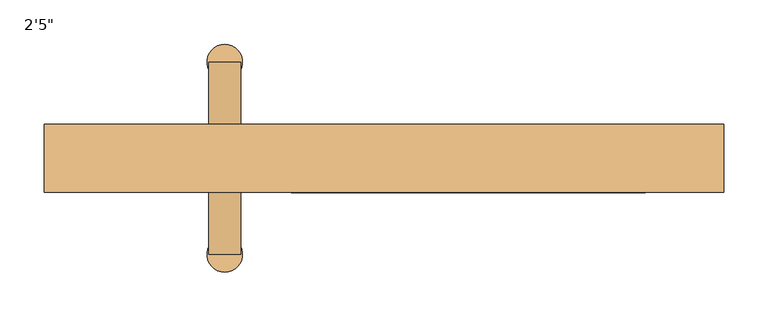
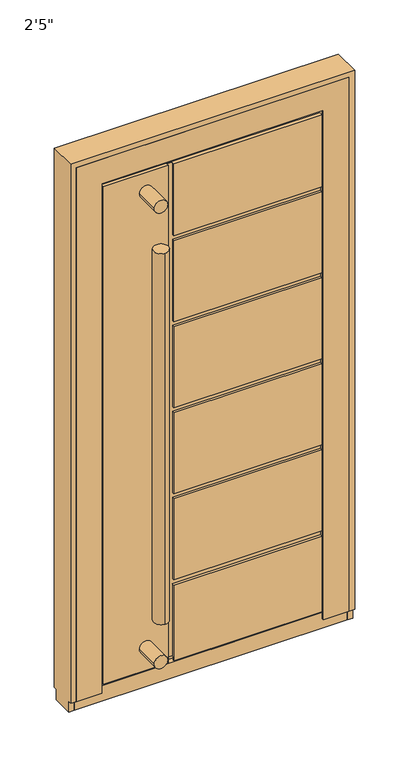
"""IFC4 building model written with IfcOpenShell, lengths in millimetres: door geometry."""

from ifc_helpers import new_model, si_unit, point, frame, frame_2d, origin, place, context, project, spatial, circle_curve, trimmed, segment, composite_curve, outline, extrude, faceted_brep, source, transform, mapped, element, save


def door_9b787682(model_context):
    return source(origin(), model_context, "Body", "SolidModel", [
        extrude(outline(composite_curve([segment(trimmed(circle_curve(frame_2d((-179.75, -90.8003001)), 20.0), [point((-179.75, -70.8003001))], [point((-179.75, -110.8003001))], False, "CARTESIAN"), True, "CONTINUOUS"), segment(trimmed(circle_curve(frame_2d((-179.75, -90.8003001)), 20.0), [point((-179.75, -110.8003001))], [point((-179.75, -70.8003001))], False, "CARTESIAN"), True, "CONTINUOUS")], self_intersect=False)), frame((0.0, 0.0, 210.0000003), z_axis=(0.0, 0.0, 1.0), x_axis=(1.0, 0.0, 0.0)), (0.0, 0.0, 1.0), 1059.0),
        extrude(outline(composite_curve([segment(trimmed(circle_curve(frame_2d((-179.75, 126.2003001)), 20.0), [point((-179.75, 146.2003001))], [point((-179.75, 106.2003001))], False, "CARTESIAN"), True, "CONTINUOUS"), segment(trimmed(circle_curve(frame_2d((-179.75, 126.2003001)), 20.0), [point((-179.75, 106.2003001))], [point((-179.75, 146.2003001))], False, "CARTESIAN"), True, "CONTINUOUS")], self_intersect=False)), frame((0.0, 0.0, 210.0000003), z_axis=(0.0, 0.0, 1.0), x_axis=(1.0, 0.0, 0.0)), (0.0, 0.0, 1.0), 1059.0),
        extrude(outline(composite_curve([segment(trimmed(circle_curve(frame_2d((89.5000003, -179.75)), 18.0), [point((89.5000003, -197.75))], [point((89.5000003, -161.75))], False, "CARTESIAN"), True, "CONTINUOUS"), segment(trimmed(circle_curve(frame_2d((89.5000003, -179.75)), 18.0), [point((89.5000003, -161.75))], [point((89.5000003, -197.75))], False, "CARTESIAN"), True, "CONTINUOUS")], self_intersect=False)), frame((0.0, -90.8, 0.0), z_axis=(0.0, 1.0, 0.0), x_axis=(0.0, 0.0, 1.0)), (0.0, 0.0, 1.0), 217.0),
        extrude(outline(composite_curve([segment(trimmed(circle_curve(frame_2d((1389.5000003, -179.75)), 18.0), [point((1389.5000003, -197.75))], [point((1389.5000003, -161.75))], False, "CARTESIAN"), True, "CONTINUOUS"), segment(trimmed(circle_curve(frame_2d((1389.5000003, -179.75)), 18.0), [point((1389.5000003, -161.75))], [point((1389.5000003, -197.75))], False, "CARTESIAN"), True, "CONTINUOUS")], self_intersect=False)), frame((0.0, -90.8, 0.0), z_axis=(0.0, 1.0, 0.0), x_axis=(0.0, 0.0, 1.0)), (0.0, 0.0, 1.0), 217.0),
        faceted_brep([(-104.75, -13.8, 255.666667), (-104.75, -13.8, 486.3333337), (294.75, -13.8, 486.3333337), (294.75, -13.8, 501.3333337), (-104.75, -13.8, 501.3333337), (-104.75, -13.8, 732.0000004), (294.75, -13.8, 732.0000004), (294.75, -13.8, 747.0000004), (-104.75, -13.8, 747.0000004), (-104.75, -13.8, 977.666667), (294.75, -13.8, 977.666667), (294.75, -13.8, 992.666667), (-104.75, -13.8, 992.666667), (-104.75, -13.8, 1223.3333337), (294.75, -13.8, 1223.3333337), (294.75, -13.8, 1238.3333337), (-104.75, -13.8, 1238.3333337), (-104.75, -13.8, 1444.0000003), (-119.75, -13.8, 1444.0000003), (-119.75, -13.8, 35.0), (-104.75, -13.8, 35.0), (-104.75, -13.8, 240.666667), (294.75, -13.8, 240.666667), (294.75, -13.8, 255.666667), (-104.75, -20.8, 255.666667), (-104.75, -20.8, 486.3333337), (294.75, -20.8, 486.3333337), (294.75, -11.7997698, 1444.0000003), (294.75, -20.8, 1444.0000003), (294.75, -20.8, 1238.3333337), (294.75, -20.8, 1223.3333337), (294.75, -20.8, 992.666667), (294.75, -20.8, 977.666667), (294.75, -20.8, 747.0000004), (294.75, -20.8, 732.0000004), (294.75, -20.8, 501.3333337), (294.75, -20.8, 255.666667), (294.75, -20.8, 240.666667), (294.75, -20.8, 24.0), (294.75, -18.8020472, 24.0), (294.75, -18.8020472, 35.0), (294.75, -11.7997698, 35.0), (-104.75, -20.8, 501.3333337), (-104.75, -20.8, 732.0000004), (-104.75, -20.8, 747.0000004), (-104.75, -20.8, 977.666667), (-119.75, -20.8, 1444.0000003), (-119.75, -20.8, 24.0), (-119.75, -18.8020472, 24.0), (-119.75, -18.8020472, 35.0), (-104.75, -18.8020472, 35.0), (-294.75, -18.8020472, 35.0), (-294.75, -11.7997698, 35.0), (-104.75, -20.8, 240.666667), (-104.75, -18.8020472, 24.0), (-104.75, -20.8, 24.0), (-294.75, -18.8020472, 24.0), (-294.75, -20.8, 24.0), (-294.75, -20.8, 1444.0000003), (-104.75, -20.8, 1223.3333337), (-104.75, -20.8, 992.666667), (-104.75, -20.8, 1444.0000003), (-104.75, -20.8, 1238.3333337), (319.75, 56.2, 10.0000003), (319.75, 53.2, 10.0000003), (-104.75, 53.2, 10.0000003), (-104.75, 56.2, 10.0000003), (-319.75, 53.2, 10.0000003), (-319.75, 56.2, 10.0000003), (-119.75, 56.2, 10.0000003), (-119.75, 53.2, 10.0000003), (319.75, 56.2, 240.666667), (319.75, 53.2, 240.666667), (319.75, 56.2, 255.666667), (319.75, 56.2, 486.3333337), (319.75, 53.2, 486.3333337), (319.75, 53.2, 255.666667), (319.75, 56.2, 747.0000004), (319.75, 56.2, 977.666667), (319.75, 53.2, 977.666667), (319.75, 53.2, 747.0000004), (319.75, 56.2, 501.3333337), (319.75, 56.2, 732.0000004), (319.75, 53.2, 732.0000004), (319.75, 53.2, 501.3333337), (319.75, 56.2, 992.666667), (319.75, 56.2, 1223.3333337), (319.75, 53.2, 1223.3333337), (319.75, 53.2, 992.666667), (319.75, 56.2, 1469.0000003), (319.75, 53.2, 1469.0000003), (319.75, 53.2, 1238.3333337), (319.75, 56.2, 1238.3333337), (304.25, 53.2, 240.666667), (304.25, 53.2, 25.5), (-104.75, 53.2, 25.5), (304.25, 53.2, 486.3333337), (304.25, 53.2, 255.666667), (304.25, 53.2, 977.666667), (304.25, 53.2, 747.0000004), (304.25, 53.2, 732.0000004), (304.25, 53.2, 501.3333337), (304.25, 53.2, 1223.3333337), (304.25, 53.2, 992.666667), (-104.75, 53.2, 1469.0000003), (-104.75, 53.2, 1453.5000003), (304.25, 53.2, 1453.5000003), (304.25, 53.2, 1238.3333337), (-304.25, 53.2, 25.5), (-304.25, 53.2, 1453.5000003), (-119.75, 53.2, 1453.5000003), (-119.75, 53.2, 1469.0000003), (-319.75, 53.2, 1469.0000003), (-119.75, 53.2, 25.5), (-104.75, 49.2, 240.666667), (-104.75, 56.2, 240.666667), (-104.75, 49.2, 25.5), (-104.75, 56.2, 255.666667), (-104.75, 56.2, 486.3333337), (-104.75, 56.2, 747.0000004), (-104.75, 56.2, 977.666667), (-104.75, 56.2, 501.3333337), (-104.75, 56.2, 732.0000004), (-104.75, 56.2, 992.666667), (-104.75, 56.2, 1223.3333337), (-104.75, 56.2, 1238.3333337), (-104.75, 56.2, 1469.0000003), (-319.75, 56.2, 1469.0000003), (-119.75, 56.2, 1469.0000003), (-119.75, 49.2, 1453.5000003), (-119.75, 49.2, 25.5), (-294.75, -11.7997698, 1444.0000003), (304.25, -11.7997698, 1453.5000003), (-304.25, -11.7997698, 1453.5000003), (-304.25, -11.7997698, 25.5), (304.25, -11.7997698, 25.5), (304.25, 49.2, 240.666667), (304.25, 49.2, 255.666667), (304.25, 49.2, 486.3333337), (304.25, 49.2, 501.3333337), (304.25, 49.2, 732.0000004), (304.25, 49.2, 747.0000004), (304.25, 49.2, 977.666667), (304.25, 49.2, 992.666667), (304.25, 49.2, 1223.3333337), (304.25, 49.2, 1238.3333337), (-104.75, 49.2, 1223.3333337), (-104.75, 49.2, 992.666667), (-104.75, 49.2, 977.666667), (-104.75, 49.2, 747.0000004), (-104.75, 49.2, 732.0000004), (-104.75, 49.2, 501.3333337), (-104.75, 49.2, 486.3333337), (-104.75, 49.2, 255.666667), (-104.75, 49.2, 1453.5000003), (-104.75, 49.2, 1238.3333337)], [[[0, 1, 2, 3, 4, 5, 6, 7, 8, 9, 10, 11, 12, 13, 14, 15, 16, 17, 18, 19, 20, 21, 22, 23]], [[1, 0, 24, 25]], [[1, 25, 26, 2]], [[27, 28, 29, 15, 14, 30, 31, 11, 10, 32, 33, 7, 6, 34, 35, 3, 2, 26, 36, 23, 22, 37, 38, 39, 40, 41]], [[42, 4, 3, 35]], [[5, 4, 42, 43]], [[5, 43, 34, 6]], [[44, 8, 7, 33]], [[9, 8, 44, 45]], [[19, 18, 46, 47, 48, 49]], [[41, 40, 50, 20, 19, 49, 51, 52]], [[53, 21, 20, 50, 54, 55]], [[21, 53, 37, 22]], [[24, 0, 23, 36]], [[40, 39, 54, 50]], [[56, 51, 49, 48]], [[39, 38, 55, 54]], [[57, 56, 48, 47]], [[33, 32, 45, 44]], [[35, 34, 43, 42]], [[36, 26, 25, 24]], [[55, 38, 37, 53]], [[58, 57, 47, 46]], [[31, 30, 59, 60]], [[28, 61, 62, 29]], [[63, 64, 65, 66]], [[67, 68, 69, 70]], [[64, 63, 71, 72]], [[73, 74, 75, 76]], [[77, 78, 79, 80]], [[81, 82, 83, 84]], [[85, 86, 87, 88]], [[89, 90, 91, 92]], [[65, 64, 72, 93, 94, 95]], [[76, 75, 96, 97]], [[80, 79, 98, 99]], [[84, 83, 100, 101]], [[88, 87, 102, 103]], [[90, 104, 105, 106, 107, 91]], [[108, 109, 110, 111, 112, 67, 70, 113]], [[114, 115, 66, 65, 95, 116]], [[63, 66, 115, 71]], [[74, 73, 117, 118]], [[78, 77, 119, 120]], [[82, 81, 121, 122]], [[86, 85, 123, 124]], [[89, 92, 125, 126]], [[68, 127, 128, 69]], [[68, 67, 112, 127]], [[129, 130, 113, 70, 69, 128, 111, 110]], [[58, 131, 52, 51, 56, 57]], [[132, 133, 134, 135], [131, 27, 41, 52]], [[106, 132, 135, 94, 93, 136, 137, 97, 96, 138, 139, 101, 100, 140, 141, 99, 98, 142, 143, 103, 102, 144, 145, 107]], [[94, 135, 134, 108, 113, 130, 116, 95]], [[133, 109, 108, 134]], [[146, 147, 143, 142, 148, 149, 141, 140, 150, 151, 139, 138, 152, 153, 137, 136, 114, 116, 130, 129, 154, 155, 145, 144]], [[149, 148, 120, 119]], [[149, 119, 77, 80, 99, 141]], [[122, 150, 140, 100, 83, 82]], [[151, 150, 122, 121]], [[151, 121, 81, 84, 101, 139]], [[118, 152, 138, 96, 75, 74]], [[153, 152, 118, 117]], [[153, 117, 73, 76, 97, 137]], [[115, 114, 136, 93, 72, 71]], [[9, 45, 32, 10]], [[60, 12, 11, 31]], [[13, 12, 60, 59]], [[13, 59, 30, 14]], [[62, 16, 15, 29]], [[16, 62, 61, 17]], [[124, 146, 144, 102, 87, 86]], [[125, 155, 154, 105, 104, 126]], [[120, 148, 142, 98, 79, 78]], [[147, 123, 85, 88, 103, 143]], [[147, 146, 124, 123]], [[155, 125, 92, 91, 107, 145]], [[90, 89, 126, 104]], [[127, 112, 111, 128]], [[132, 106, 105, 154, 129, 110, 109, 133]], [[27, 131, 58, 46, 18, 17, 61, 28]]]),
        faceted_brep([(-368.3, 56.2, 0.0), (-323.8, 56.2, 0.0), (-323.8, 47.2, 0.0), (-368.3, 47.1997571, 0.0), (-314.3, -16.2999958, 0.0), (-298.8, -16.2999958, 0.0), (-298.8, -20.8, 0.0), (-368.3, -20.8, 0.0), (-368.3, -11.8, 0.0), (-314.3, -11.8, 0.0), (368.3, -20.8, 0.0), (298.8, -20.8, 0.0), (298.8, -16.2999958, 0.0), (314.3, -16.2999958, 0.0), (314.3, -11.8, 0.0), (368.3, -11.8, 0.0), (323.8, 47.2, 0.0), (323.8, 56.2, 0.0), (368.3, 56.2, 0.0), (368.3, 47.1997571, 0.0), (-368.3, -20.8, 1524.0), (-368.3, 56.2, 1524.0), (-368.3, 47.1997571, -30.0), (-368.3, -11.8, -30.0), (368.3, 56.2, 1524.0), (323.8, 56.2, 1479.5), (-323.8, 56.2, 1479.5), (368.3, -20.8, 1524.0), (368.3, -11.8, -30.0), (368.3, 47.1997571, -30.0), (-298.8, -20.8, 1454.5), (298.8, -20.8, 1454.5), (-314.3, 47.2, 1470.0), (-314.3, -16.2999958, 1470.0), (-314.3, -11.8, 14.5), (-314.3, 47.2, 14.5), (314.3, 47.2, 1470.0), (314.3, -16.2999958, 1470.0), (314.3, 47.2, 14.5), (314.3, -11.8, 14.5), (-323.8, 47.2, 1479.5), (323.8, 47.2, 1479.5), (298.8, -16.2999958, 1454.5), (-298.8, -16.2999958, 1454.5)], [[[0, 1, 2, 3]], [[4, 5, 6, 7, 8, 9]], [[10, 11, 12, 13, 14, 15]], [[16, 17, 18, 19]], [[7, 20, 21, 0, 3, 22, 23, 8]], [[1, 0, 21, 24, 18, 17, 25, 26]], [[21, 20, 27, 24]], [[18, 24, 27, 10, 15, 28, 29, 19]], [[7, 6, 30, 31, 11, 10, 27, 20]], [[32, 33, 4, 9, 34, 35]], [[33, 32, 36, 37]], [[37, 36, 38, 39, 14, 13]], [[40, 2, 1, 26]], [[16, 19, 29, 22, 3, 2, 40, 41], [36, 32, 35, 38]], [[5, 4, 33, 37, 13, 12, 42, 43]], [[6, 5, 43, 30]], [[26, 25, 41, 40]], [[31, 30, 43, 42]], [[17, 16, 41, 25]], [[12, 11, 31, 42]], [[23, 28, 15, 14, 39, 34, 9, 8]], [[38, 35, 34, 39]], [[23, 22, 29, 28]]]),
        faceted_brep([(-368.3, 47.2, -30.0), (-368.3, -11.8, -30.0), (-383.3, -11.8, -30.0), (-383.3, 47.2, -30.0), (-368.3, 56.2, 1524.0), (-368.3, -20.8, 1524.0), (-368.3, -20.8, 0.0), (-368.3, -11.8, 0.0), (-368.3, 47.2, 0.0), (-368.3, 56.2, 0.0), (383.3, -11.8, 0.0), (368.3, -11.8, 0.0), (368.3, -11.8, -30.0), (383.3, -11.8, -30.0), (-383.3, -11.8, 0.0), (-383.3, -20.8, 1539.0), (-383.3, 56.2, 1539.0), (-383.3, 56.2, 0.0), (-383.3, 47.2, 0.0), (-383.3, -20.8, 0.0), (368.3, 47.2, 0.0), (383.3, 47.2, 0.0), (383.3, 47.2, -30.0), (368.3, 47.2, -30.0), (368.3, -20.8, 1524.0), (368.3, 56.2, 1524.0), (368.3, 56.2, 0.0), (368.3, -20.8, 0.0), (383.3, 56.2, 1539.0), (383.3, 56.2, 0.0), (383.3, -20.8, 0.0), (383.3, -20.8, 1539.0)], [[[0, 1, 2, 3]], [[4, 5, 6, 7, 1, 0, 8, 9]], [[10, 11, 12, 13]], [[7, 14, 2, 1]], [[15, 16, 17, 18, 3, 2, 14, 19]], [[20, 21, 22, 23]], [[18, 8, 0, 3]], [[24, 25, 26, 20, 23, 12, 11, 27]], [[25, 4, 9, 17, 16, 28, 29, 26]], [[21, 20, 26, 29]], [[8, 18, 17, 9]], [[22, 13, 12, 23]], [[11, 10, 30, 27]], [[14, 7, 6, 19]], [[5, 24, 27, 30, 31, 15, 19, 6]], [[28, 31, 30, 10, 13, 22, 21, 29]], [[5, 4, 25, 24]], [[16, 15, 31, 28]]]),
    ])


if __name__ == "__main__":
    model = new_model("IFC4")
    model_context = context("Model", 3, world=origin())
    ifc_project = project(units=[si_unit("LENGTHUNIT", "METRE", prefix="MILLI")], contexts=[model_context])
    site = spatial("IfcSite", under=ifc_project)
    building = spatial("IfcBuilding", under=site)
    placement = place(None, origin())
    door_shape = door_9b787682(model_context)
    element("IfcDoor", 1, ObjectType="2'5\"", at=placement, inside=building, context=model_context, shape_type="MappedRepresentation", body=[
        mapped(door_shape, transform((0.0, 0.0, 0.0), x_axis=(1.0, 0.0, 0.0), y_axis=(0.0, 1.0, 0.0), z_axis=(0.0, 0.0, 1.0))),
    ])
    save(model, "model.ifc")

# Revit data of these elements
# Type "2'5\""
#   Type Mark = "9"
#   Water resistance = "up to Class E900, EN 12208:2001"
#   Uniclass2015Version = "v1.21"
#   Uniclass2015Reference = "Ss_25_30_20_30"
#   Uniclass2015Description = "Frame and door leaf system"
#   URL = "www.aluprof.com"
#   Type IFC Predefined Type = "USERDEFINED"
#   Right-hand / Left-hand door [instance default] = ""
#   Resistance to wind load = "up to Class C5/B5, EN 12210:2001"
#   Insert type = "ST"
#   Hardware [instance default] = ""
#   Product page = "https://aluprof.com/en/architects/offer/window-and-door-systems/panel-doors#visualisation"
#   Operation = "SinglePanelOutwardOpening"
#   Opening type = "Outward"
#   NBSReference = "25-50-20/125"
#   NBSDescription = "Frame and door leaf system"
#   Important = "The actual acceptable construction dimensions are dependent on the selection of profiles and hardware, glazing type, construction weight and the construction’s operating conditions. These should be determined by a suitably qualified person, and using ALUPROF’s calculation software"
#   IfcExportType = "USERDEFINED"
#   IfcExportAs = "IfcDoorType"
#   Handle type [instance default] = ""
#   Manufacturer = "ALUPROF SA"
#   Export Type to IFC As = "IfcDoorType"
#   Door sill type [instance default] = ""
#   Description = "External single-leaf panel door outward opening"
#   Model = "MB-86 ST Panel Door AD07"
#   Content of the recyclate in the material = "69.2%"
#   COBie.Type.WarrantyDurationParts = ""
#   COBie.Type.Name = ""
#   COBie.Type.Manufacturer = "ALUPROF SA"
#   COBie.Space.Name = ""
#   COBie.Floor.Name = ""
#   COBie.Facility.Name = ""
#   COBie.CreatedOn = ""
#   COBie.Component.WarrantyStartDate = ""
#   COBie.Component.Name = "MB-86 ST Panel Door AD07"
#   Burglar resistance = "RC2"
#   Air permeability = "up to Class 4, EN 12207:2001"
#   Width of the active leaf = 2' - 1.17717"
#   Placement in wall = 0' - 0.7874"
#   Thickness = 0' - 3.0315"
#   Height of the opening sash = 4' - 9.44094"
#   Handle Offset = 3' - 5.33858"
#   Rough Height = 5' - 2.40945"
#   Rough Width = 2' - 6.1811"
#   Height = 5' - 0"
#   Width = 2' - 5"
#   Construction depth = 0' - 3.0315"
#   Clear opening width = 1' - 8.94882"
#   Clear opening height = 4' - 8.47638"
#   Height of the array = 0' - 9.08136"
#   Schedule No. [instance default] = 1
#   Handrail [instance default] = yes
#   IsExternal = yes
#   Handle [instance default] = no
#   Door closer [instance default] = no
#   Function = 1
#   COBie.Type = yes
#   COBie = yes
#   Access control [instance default] = no
#   Panel = element 346771
#   Wall Closure = (empty or 0)
